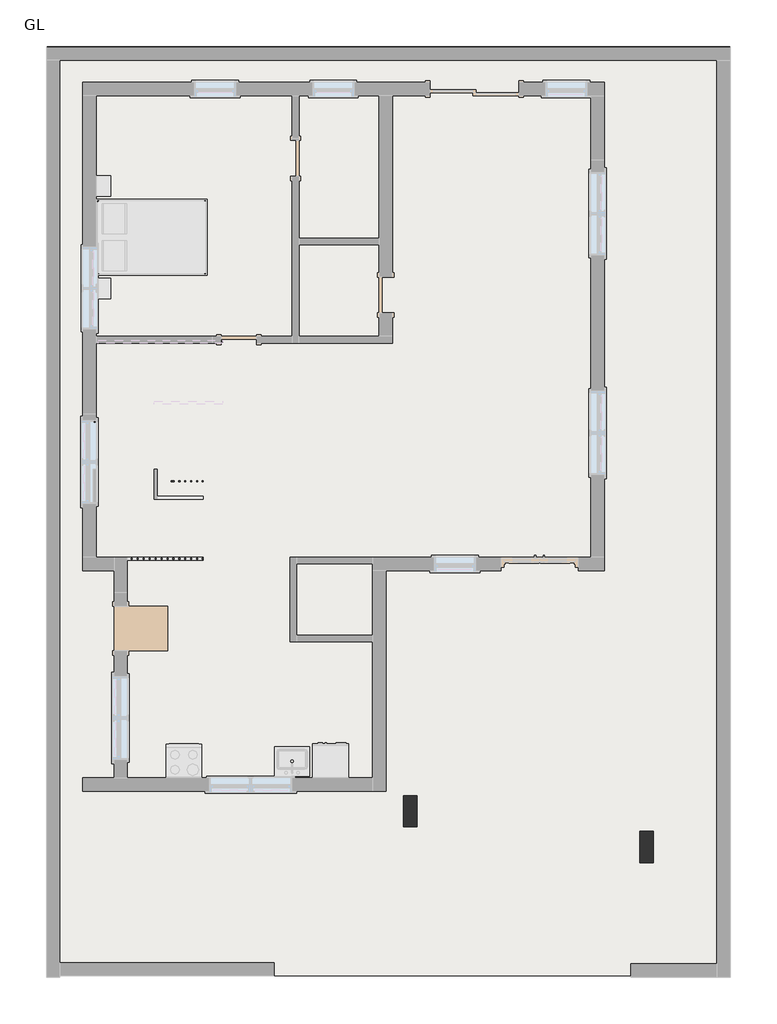
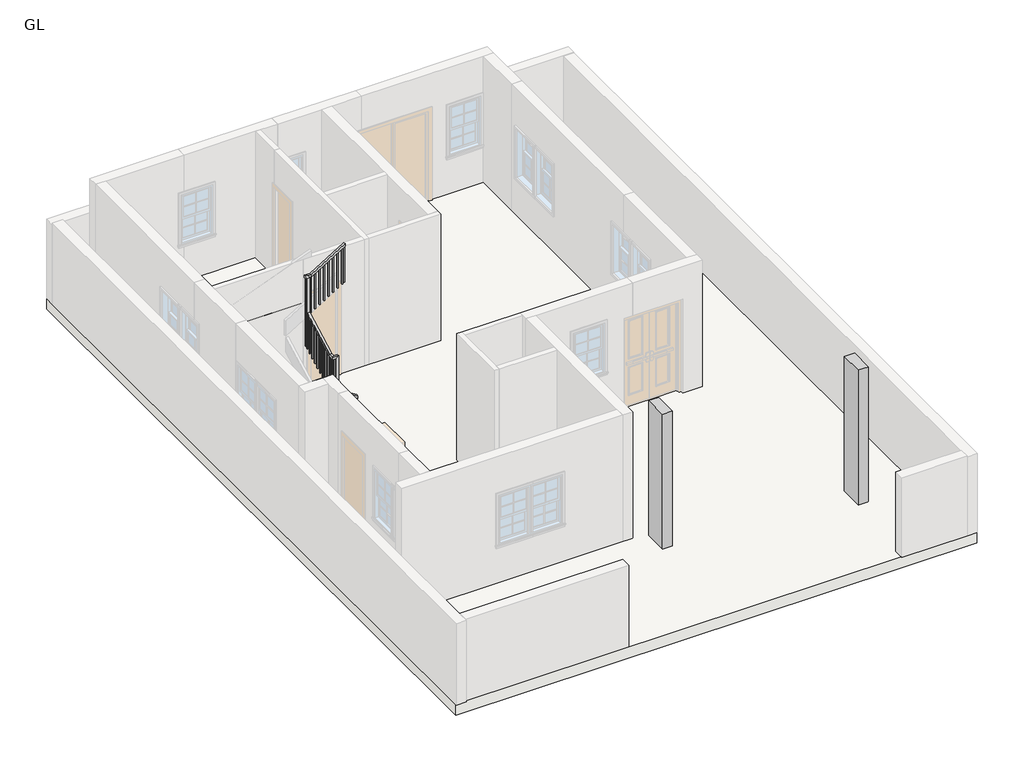
# One storey, part 2 of 3: 2 columns, 2 railings, 1 slab.
"""IFC4 building model written with IfcOpenShell, lengths in millimetres."""

from ifc_helpers import new_model, si_unit, frame, origin, place, context, project, spatial, polyline, outline, extrude, faceted_brep, transform, mapped, element, save
from components import column_1de33f28

model = new_model("IFC4")

# Units and contexts
model_context = context("Model", 3, world=origin())
ifc_project = project(units=[si_unit("LENGTHUNIT", "METRE", prefix="MILLI")], contexts=[model_context])

# Site, building, storey
site = spatial("IfcSite", under=ifc_project)
building = spatial("IfcBuilding", under=site)
storey = spatial("IfcBuildingStorey", under=building, Name="GL", Elevation=0.0)

# Columns
placement = place(None, origin())
column_shape = column_1de33f28(model_context)
element("IfcColumn", 1, ObjectType="Rectangular Column : x9\"", at=placement, inside=storey, context=model_context, shape_type="MappedRepresentation", body=[
    mapped(column_shape, transform((-16875.4750314, 319.9223646, 0.0), x_axis=(1.0, 0.0, 0.0), y_axis=(0.0, 1.0, 0.0), z_axis=(0.0, 0.0, 1.0))),
])
element("IfcColumn", 2, ObjectType="Rectangular Column : x9\"", at=placement, inside=storey, context=model_context, shape_type="MappedRepresentation", body=[
    mapped(column_shape, transform((-12836.8750314, -289.6776354, 0.0), x_axis=(1.0, 0.0, 0.0), y_axis=(0.0, 1.0, 0.0), z_axis=(0.0, 0.0, 1.0))),
])

# Railings
element("IfcRailing", 3, ObjectType="Handrail - Rectangular", at=placement, inside=storey, context=model_context, shape_type="SolidModel", body=[
    faceted_brep([(-20418.7750314, 5933.3223646, 1270.0), (-20418.7750314, 5933.3223646, 1209.786276), (-20418.7750314, 5984.1223646, 1209.786276), (-20418.7750314, 5984.1223646, 1270.0), (-20850.5750314, 5933.3223646, 1544.7818182), (-20901.3750314, 5933.3223646, 1516.8953669), (-20901.3750314, 5984.1223646, 1516.8953669), (-20850.5750314, 5984.1223646, 1544.7818182), (-20850.5750314, 5933.3223646, 2374.5151515), (-20901.3750314, 5933.3223646, 2323.7151515), (-20901.3750314, 5984.1223646, 2323.7151515), (-20850.5750314, 5984.1223646, 2374.5151515), (-20977.5750314, 5933.3223646, 2374.5151515), (-20977.5750314, 5933.3223646, 2323.7151515), (-20926.7750314, 5984.1223646, 2323.7151515), (-20926.7750314, 5984.1223646, 2374.5151515), (-20977.5750314, 6060.3223646, 2374.5151515), (-20977.5750314, 6072.9586335, 2323.7151515), (-20926.7750314, 6072.9586335, 2323.7151515), (-20926.7750314, 6060.3223646, 2374.5151515), (-20977.5750314, 6923.9223646, 2832.4848485), (-20977.5750314, 6974.7223646, 2801.9231907), (-20926.7750314, 6974.7223646, 2801.9231907), (-20926.7750314, 6923.9223646, 2832.4848485), (-20088.5750314, 7050.9223646, 4114.8), (-20088.5750314, 7000.1223646, 4114.8), (-20088.5750314, 7000.1223646, 4055.3290495), (-20088.5750314, 7050.9223646, 4055.3290495), (-20836.3298984, 7050.9223646, 3600.173913), (-20850.5750314, 7050.9223646, 3650.973913), (-20836.3298984, 7000.1223646, 3600.173913), (-20850.5750314, 7000.1223646, 3650.973913), (-20977.5750314, 6923.9223646, 3650.973913), (-20977.5750314, 6974.7223646, 3600.173913), (-20926.7750314, 6974.7223646, 3600.173913), (-20926.7750314, 6923.9223646, 3650.973913), (-20977.5750314, 7050.9223646, 3650.973913), (-20977.5750314, 7050.9223646, 3600.173913), (-20926.7750314, 7000.1223646, 3600.173913), (-20926.7750314, 7000.1223646, 3650.973913)], [[[0, 1, 2, 3]], [[1, 0, 4, 5]], [[2, 1, 5, 6]], [[3, 2, 6, 7]], [[0, 3, 7, 4]], [[5, 4, 8, 9]], [[6, 5, 9, 10]], [[7, 6, 10, 11]], [[4, 7, 11, 8]], [[9, 8, 12, 13]], [[10, 9, 13, 14]], [[11, 10, 14, 15]], [[8, 11, 15, 12]], [[13, 12, 16, 17]], [[14, 13, 17, 18]], [[15, 14, 18, 19]], [[12, 15, 19, 16]], [[17, 16, 20, 21]], [[18, 17, 21, 22]], [[19, 18, 22, 23]], [[16, 19, 23, 20]], [[24, 25, 26, 27]], [[28, 29, 24, 27]], [[30, 28, 27, 26]], [[31, 30, 26, 25]], [[29, 31, 25, 24]], [[21, 20, 32, 33]], [[22, 21, 33, 34]], [[23, 22, 34, 35]], [[20, 23, 35, 32]], [[33, 32, 36, 37]], [[34, 33, 37, 38]], [[35, 34, 38, 39]], [[32, 35, 39, 36]], [[37, 36, 29, 28]], [[38, 37, 28, 30]], [[39, 38, 30, 31]], [[36, 39, 31, 29]]]),
    extrude(outline(polyline([(4030.2051365, -20129.8500314), (4018.6094843, -20148.9000314), (3169.4782609, -20148.9000314), (3169.4782609, -20129.8500314), (4030.2051365, -20129.8500314)])), frame((0.0, 7015.9973646, 0.0), z_axis=(0.0, 1.0, 0.0), x_axis=(0.0, 0.0, 1.0)), (0.0, 0.0, 1.0), 19.05),
    extrude(outline(polyline([(3968.3616582, -20231.4500314), (3956.766006, -20250.5000314), (3107.6347826, -20250.5000314), (3107.6347826, -20231.4500314), (3968.3616582, -20231.4500314)])), frame((0.0, 7015.9973646, 0.0), z_axis=(0.0, 1.0, 0.0), x_axis=(0.0, 0.0, 1.0)), (0.0, 0.0, 1.0), 19.05),
    extrude(outline(polyline([(3906.51818, -20333.0500314), (3894.9225278, -20352.1000314), (3045.7913043, -20352.1000314), (3045.7913043, -20333.0500314), (3906.51818, -20333.0500314)])), frame((0.0, 7015.9973646, 0.0), z_axis=(0.0, 1.0, 0.0), x_axis=(0.0, 0.0, 1.0)), (0.0, 0.0, 1.0), 19.05),
    extrude(outline(polyline([(3844.6747017, -20434.6500314), (3833.0790495, -20453.7000314), (2983.9478261, -20453.7000314), (2983.9478261, -20434.6500314), (3844.6747017, -20434.6500314)])), frame((0.0, 7015.9973646, 0.0), z_axis=(0.0, 1.0, 0.0), x_axis=(0.0, 0.0, 1.0)), (0.0, 0.0, 1.0), 19.05),
    extrude(outline(polyline([(3782.8312234, -20536.2500314), (3771.2355713, -20555.3000314), (2922.1043478, -20555.3000314), (2922.1043478, -20536.2500314), (3782.8312234, -20536.2500314)])), frame((0.0, 7015.9973646, 0.0), z_axis=(0.0, 1.0, 0.0), x_axis=(0.0, 0.0, 1.0)), (0.0, 0.0, 1.0), 19.05),
    extrude(outline(polyline([(3720.9877452, -20637.8500314), (3709.392093, -20656.9000314), (2860.2608696, -20656.9000314), (2860.2608696, -20637.8500314), (3720.9877452, -20637.8500314)])), frame((0.0, 7015.9973646, 0.0), z_axis=(0.0, 1.0, 0.0), x_axis=(0.0, 0.0, 1.0)), (0.0, 0.0, 1.0), 19.05),
    extrude(outline(polyline([(3659.1442669, -20739.4500314), (3647.5486147, -20758.5000314), (2798.4173913, -20758.5000314), (2798.4173913, -20739.4500314), (3659.1442669, -20739.4500314)])), frame((0.0, 7015.9973646, 0.0), z_axis=(0.0, 1.0, 0.0), x_axis=(0.0, 0.0, 1.0)), (0.0, 0.0, 1.0), 19.05),
    extrude(outline(polyline([(3597.3007887, -20841.0500314), (3585.7051365, -20860.1000314), (2736.573913, -20860.1000314), (2736.573913, -20841.0500314), (3597.3007887, -20841.0500314)])), frame((0.0, 7015.9973646, 0.0), z_axis=(0.0, 1.0, 0.0), x_axis=(0.0, 0.0, 1.0)), (0.0, 0.0, 1.0), 19.05),
    extrude(outline(polyline([(-20942.6500314, 6965.1973646), (-20961.7000314, 6965.1973646), (-20961.7000314, 6984.2473646), (-20942.6500314, 6984.2473646), (-20942.6500314, 6965.1973646)])), frame((0.0, 0.0, 1945.0242424), z_axis=(0.0, 0.0, 1.0), x_axis=(1.0, 0.0, 0.0)), (0.0, 0.0, 1.0), 1655.1496706),
    extrude(outline(polyline([(6863.5973646, 2742.9932665), (6882.6473646, 2753.0955392), (6882.6473646, 1891.1454545), (6863.5973646, 1891.1454545), (6863.5973646, 2742.9932665)])), frame((-20961.7000314, 0.0, 0.0), z_axis=(1.0, 0.0, 0.0), x_axis=(0.0, 1.0, 0.0)), (0.0, 0.0, 1.0), 19.05),
    extrude(outline(polyline([(6761.9973646, 2689.1144786), (6781.0473646, 2699.2167513), (6781.0473646, 1837.2666667), (6761.9973646, 1837.2666667), (6761.9973646, 2689.1144786)])), frame((-20961.7000314, 0.0, 0.0), z_axis=(1.0, 0.0, 0.0), x_axis=(0.0, 1.0, 0.0)), (0.0, 0.0, 1.0), 19.05),
    extrude(outline(polyline([(6660.3973646, 2635.2356907), (6679.4473646, 2645.3379635), (6679.4473646, 1783.3878788), (6660.3973646, 1783.3878788), (6660.3973646, 2635.2356907)])), frame((-20961.7000314, 0.0, 0.0), z_axis=(1.0, 0.0, 0.0), x_axis=(0.0, 1.0, 0.0)), (0.0, 0.0, 1.0), 19.05),
    extrude(outline(polyline([(6558.7973646, 2581.3569029), (6577.8473646, 2591.4591756), (6577.8473646, 1729.5090909), (6558.7973646, 1729.5090909), (6558.7973646, 2581.3569029)])), frame((-20961.7000314, 0.0, 0.0), z_axis=(1.0, 0.0, 0.0), x_axis=(0.0, 1.0, 0.0)), (0.0, 0.0, 1.0), 19.05),
    extrude(outline(polyline([(6457.1973646, 2527.478115), (6476.2473646, 2537.5803877), (6476.2473646, 1675.630303), (6457.1973646, 1675.630303), (6457.1973646, 2527.478115)])), frame((-20961.7000314, 0.0, 0.0), z_axis=(1.0, 0.0, 0.0), x_axis=(0.0, 1.0, 0.0)), (0.0, 0.0, 1.0), 19.05),
    extrude(outline(polyline([(6355.5973646, 2473.5993271), (6374.6473646, 2483.7015998), (6374.6473646, 1621.7515152), (6355.5973646, 1621.7515152), (6355.5973646, 2473.5993271)])), frame((-20961.7000314, 0.0, 0.0), z_axis=(1.0, 0.0, 0.0), x_axis=(0.0, 1.0, 0.0)), (0.0, 0.0, 1.0), 19.05),
    extrude(outline(polyline([(6253.9973646, 2419.7205392), (6273.0473646, 2429.8228119), (6273.0473646, 1567.8727273), (6253.9973646, 1567.8727273), (6253.9973646, 2419.7205392)])), frame((-20961.7000314, 0.0, 0.0), z_axis=(1.0, 0.0, 0.0), x_axis=(0.0, 1.0, 0.0)), (0.0, 0.0, 1.0), 19.05),
    extrude(outline(polyline([(6152.3973646, 2365.8417513), (6171.4473646, 2375.9440241), (6171.4473646, 1513.9939394), (6152.3973646, 1513.9939394), (6152.3973646, 2365.8417513)])), frame((-20961.7000314, 0.0, 0.0), z_axis=(1.0, 0.0, 0.0), x_axis=(0.0, 1.0, 0.0)), (0.0, 0.0, 1.0), 19.05),
    extrude(outline(polyline([(6050.7973646, 2311.9629635), (6069.8473646, 2322.0652362), (6069.8473646, 1460.1151515), (6050.7973646, 1460.1151515), (6050.7973646, 2311.9629635)])), frame((-20961.7000314, 0.0, 0.0), z_axis=(1.0, 0.0, 0.0), x_axis=(0.0, 1.0, 0.0)), (0.0, 0.0, 1.0), 19.05),
    extrude(outline(polyline([(-20917.2500314, 5968.2473646), (-20917.2500314, 5949.1973646), (-20936.3000314, 5949.1973646), (-20936.3000314, 5968.2473646), (-20917.2500314, 5968.2473646)])), frame((0.0, 0.0, 678.8727273), z_axis=(0.0, 0.0, 1.0), x_axis=(1.0, 0.0, 0.0)), (0.0, 0.0, 1.0), 1644.8424242),
    extrude(outline(polyline([(1462.3430941, -20815.6500314), (1474.4658214, -20834.7000314), (614.2181818, -20834.7000314), (614.2181818, -20815.6500314), (1462.3430941, -20815.6500314)])), frame((0.0, 5949.1973646, 0.0), z_axis=(0.0, 1.0, 0.0), x_axis=(0.0, 0.0, 1.0)), (0.0, 0.0, 1.0), 19.05),
    extrude(outline(polyline([(1397.6885487, -20714.0500314), (1409.811276, -20733.1000314), (549.5636364, -20733.1000314), (549.5636364, -20714.0500314), (1397.6885487, -20714.0500314)])), frame((0.0, 5949.1973646, 0.0), z_axis=(0.0, 1.0, 0.0), x_axis=(0.0, 0.0, 1.0)), (0.0, 0.0, 1.0), 19.05),
    extrude(outline(polyline([(1333.0340032, -20612.4500314), (1345.1567305, -20631.5000314), (484.9090909, -20631.5000314), (484.9090909, -20612.4500314), (1333.0340032, -20612.4500314)])), frame((0.0, 5949.1973646, 0.0), z_axis=(0.0, 1.0, 0.0), x_axis=(0.0, 0.0, 1.0)), (0.0, 0.0, 1.0), 19.05),
    extrude(outline(polyline([(1268.3794578, -20510.8500314), (1280.5021851, -20529.9000314), (420.2545455, -20529.9000314), (420.2545455, -20510.8500314), (1268.3794578, -20510.8500314)])), frame((0.0, 5949.1973646, 0.0), z_axis=(0.0, 1.0, 0.0), x_axis=(0.0, 0.0, 1.0)), (0.0, 0.0, 1.0), 19.05),
    extrude(outline(polyline([(-20942.6500314, 7015.9973646), (-20961.7000314, 7015.9973646), (-20961.7000314, 7035.0473646), (-20942.6500314, 7035.0473646), (-20942.6500314, 7015.9973646)])), frame((0.0, 0.0, 1971.9636364), z_axis=(0.0, 0.0, 1.0), x_axis=(1.0, 0.0, 0.0)), (0.0, 0.0, 1.0), 1628.2102767),
    extrude(outline(polyline([(-20942.6500314, 5968.2473646), (-20942.6500314, 5949.1973646), (-20961.7000314, 5949.1973646), (-20961.7000314, 5968.2473646), (-20942.6500314, 5968.2473646)])), frame((0.0, 0.0, 695.0363636), z_axis=(0.0, 0.0, 1.0), x_axis=(1.0, 0.0, 0.0)), (0.0, 0.0, 1.0), 1628.6787879),
    extrude(outline(polyline([(4055.3290495, -20088.5750314), (4043.7333973, -20107.6250314), (3194.6021739, -20107.6250314), (3194.6021739, -20088.5750314), (4055.3290495, -20088.5750314)])), frame((0.0, 7015.9973646, 0.0), z_axis=(0.0, 1.0, 0.0), x_axis=(0.0, 0.0, 1.0)), (0.0, 0.0, 1.0), 19.05),
    extrude(outline(polyline([(1209.786276, -20418.7750314), (1221.9090032, -20437.8250314), (361.6613636, -20437.8250314), (361.6613636, -20418.7750314), (1209.786276, -20418.7750314)])), frame((0.0, 5949.1973646, 0.0), z_axis=(0.0, 1.0, 0.0), x_axis=(0.0, 0.0, 1.0)), (0.0, 0.0, 1.0), 19.05),
])
element("IfcRailing", 4, ObjectType="Handrail - Rectangular", at=placement, inside=storey, context=model_context, shape_type="SolidModel", body=[
    faceted_brep([(-20418.7750314, 4612.5223646, 1270.0), (-20418.7750314, 4612.5223646, 1215.4938354), (-20418.7750314, 4663.3223646, 1215.4938354), (-20418.7750314, 4663.3223646, 1270.0), (-22171.3752061, 4612.5223646, 1951.5667346), (-22222.1752061, 4612.5223646, 1916.8161256), (-22222.1752061, 4663.3223646, 1916.8161256), (-22171.3752061, 4663.3223646, 1951.5667346), (-22171.3752061, 4612.5223646, 1981.200068), (-22222.1752061, 4612.5223646, 1930.400068), (-22222.1752061, 4663.3223646, 1930.400068), (-22171.3752061, 4663.3223646, 1981.200068), (-22298.3752061, 4612.5223646, 1981.200068), (-22298.3752061, 4612.5223646, 1930.400068), (-22247.5752061, 4663.3223646, 1930.400068), (-22247.5752061, 4663.3223646, 1981.200068), (-22298.3752061, 4739.5223646, 1981.200068), (-22298.3752061, 4739.5223646, 1930.400068), (-22247.5752061, 4739.5223646, 1930.400068), (-22247.5752061, 4739.5223646, 1981.200068), (-22298.3752061, 8371.7223646, 1981.200068), (-22298.3752061, 8371.7223646, 1930.400068), (-22247.5752061, 8320.9223646, 1930.400068), (-22247.5752061, 8320.9223646, 1981.200068), (-20088.5750314, 8371.7223646, 1981.200068), (-20088.5750314, 8320.9223646, 1981.200068), (-20088.5750314, 8320.9223646, 1930.400068), (-20088.5750314, 8371.7223646, 1930.400068)], [[[0, 1, 2, 3]], [[1, 0, 4, 5]], [[2, 1, 5, 6]], [[3, 2, 6, 7]], [[0, 3, 7, 4]], [[5, 4, 8, 9]], [[6, 5, 9, 10]], [[7, 6, 10, 11]], [[4, 7, 11, 8]], [[9, 8, 12, 13]], [[10, 9, 13, 14]], [[11, 10, 14, 15]], [[8, 11, 15, 12]], [[13, 12, 16, 17]], [[14, 13, 17, 18]], [[15, 14, 18, 19]], [[12, 15, 19, 16]], [[17, 16, 20, 21]], [[18, 17, 21, 22]], [[19, 18, 22, 23]], [[16, 19, 23, 20]], [[24, 25, 26, 27]], [[21, 20, 24, 27]], [[22, 21, 27, 26]], [[23, 22, 26, 25]], [[20, 23, 25, 24]]]),
    extrude(outline(polyline([(-20148.9002061, 8355.8473646), (-20129.8502061, 8355.8473646), (-20129.8502061, 8336.7973646), (-20148.9002061, 8336.7973646), (-20148.9002061, 8355.8473646)])), frame((0.0, 0.0, 1066.800068), z_axis=(0.0, 0.0, 1.0), x_axis=(1.0, 0.0, 0.0)), (0.0, 0.0, 1.0), 863.6),
    extrude(outline(polyline([(-20250.5002061, 8355.8473646), (-20231.4502061, 8355.8473646), (-20231.4502061, 8336.7973646), (-20250.5002061, 8336.7973646), (-20250.5002061, 8355.8473646)])), frame((0.0, 0.0, 1066.800068), z_axis=(0.0, 0.0, 1.0), x_axis=(1.0, 0.0, 0.0)), (0.0, 0.0, 1.0), 863.6),
    extrude(outline(polyline([(-20352.1002061, 8355.8473646), (-20333.0502061, 8355.8473646), (-20333.0502061, 8336.7973646), (-20352.1002061, 8336.7973646), (-20352.1002061, 8355.8473646)])), frame((0.0, 0.0, 1066.800068), z_axis=(0.0, 0.0, 1.0), x_axis=(1.0, 0.0, 0.0)), (0.0, 0.0, 1.0), 863.6),
    extrude(outline(polyline([(-20453.7002061, 8355.8473646), (-20434.6502061, 8355.8473646), (-20434.6502061, 8336.7973646), (-20453.7002061, 8336.7973646), (-20453.7002061, 8355.8473646)])), frame((0.0, 0.0, 1066.800068), z_axis=(0.0, 0.0, 1.0), x_axis=(1.0, 0.0, 0.0)), (0.0, 0.0, 1.0), 863.6),
    extrude(outline(polyline([(-20555.3002061, 8355.8473646), (-20536.2502061, 8355.8473646), (-20536.2502061, 8336.7973646), (-20555.3002061, 8336.7973646), (-20555.3002061, 8355.8473646)])), frame((0.0, 0.0, 1066.800068), z_axis=(0.0, 0.0, 1.0), x_axis=(1.0, 0.0, 0.0)), (0.0, 0.0, 1.0), 863.6),
    extrude(outline(polyline([(-20656.9002061, 8355.8473646), (-20637.8502061, 8355.8473646), (-20637.8502061, 8336.7973646), (-20656.9002061, 8336.7973646), (-20656.9002061, 8355.8473646)])), frame((0.0, 0.0, 1066.800068), z_axis=(0.0, 0.0, 1.0), x_axis=(1.0, 0.0, 0.0)), (0.0, 0.0, 1.0), 863.6),
    extrude(outline(polyline([(-20758.5002061, 8355.8473646), (-20739.4502061, 8355.8473646), (-20739.4502061, 8336.7973646), (-20758.5002061, 8336.7973646), (-20758.5002061, 8355.8473646)])), frame((0.0, 0.0, 1066.800068), z_axis=(0.0, 0.0, 1.0), x_axis=(1.0, 0.0, 0.0)), (0.0, 0.0, 1.0), 863.6),
    extrude(outline(polyline([(-20860.1002061, 8355.8473646), (-20841.0502061, 8355.8473646), (-20841.0502061, 8336.7973646), (-20860.1002061, 8336.7973646), (-20860.1002061, 8355.8473646)])), frame((0.0, 0.0, 1066.800068), z_axis=(0.0, 0.0, 1.0), x_axis=(1.0, 0.0, 0.0)), (0.0, 0.0, 1.0), 863.6),
    extrude(outline(polyline([(-20961.7002061, 8355.8473646), (-20942.6502061, 8355.8473646), (-20942.6502061, 8336.7973646), (-20961.7002061, 8336.7973646), (-20961.7002061, 8355.8473646)])), frame((0.0, 0.0, 1066.800068), z_axis=(0.0, 0.0, 1.0), x_axis=(1.0, 0.0, 0.0)), (0.0, 0.0, 1.0), 863.6),
    extrude(outline(polyline([(-21063.3002061, 8355.8473646), (-21044.2502061, 8355.8473646), (-21044.2502061, 8336.7973646), (-21063.3002061, 8336.7973646), (-21063.3002061, 8355.8473646)])), frame((0.0, 0.0, 1066.800068), z_axis=(0.0, 0.0, 1.0), x_axis=(1.0, 0.0, 0.0)), (0.0, 0.0, 1.0), 863.6),
    extrude(outline(polyline([(-21164.9002061, 8355.8473646), (-21145.8502061, 8355.8473646), (-21145.8502061, 8336.7973646), (-21164.9002061, 8336.7973646), (-21164.9002061, 8355.8473646)])), frame((0.0, 0.0, 1066.800068), z_axis=(0.0, 0.0, 1.0), x_axis=(1.0, 0.0, 0.0)), (0.0, 0.0, 1.0), 863.6),
    extrude(outline(polyline([(-21266.5002061, 8355.8473646), (-21247.4502061, 8355.8473646), (-21247.4502061, 8336.7973646), (-21266.5002061, 8336.7973646), (-21266.5002061, 8355.8473646)])), frame((0.0, 0.0, 1066.800068), z_axis=(0.0, 0.0, 1.0), x_axis=(1.0, 0.0, 0.0)), (0.0, 0.0, 1.0), 863.6),
    extrude(outline(polyline([(-21368.1002061, 8355.8473646), (-21349.0502061, 8355.8473646), (-21349.0502061, 8336.7973646), (-21368.1002061, 8336.7973646), (-21368.1002061, 8355.8473646)])), frame((0.0, 0.0, 1066.800068), z_axis=(0.0, 0.0, 1.0), x_axis=(1.0, 0.0, 0.0)), (0.0, 0.0, 1.0), 863.6),
    extrude(outline(polyline([(-21469.7002061, 8355.8473646), (-21450.6502061, 8355.8473646), (-21450.6502061, 8336.7973646), (-21469.7002061, 8336.7973646), (-21469.7002061, 8355.8473646)])), frame((0.0, 0.0, 1066.800068), z_axis=(0.0, 0.0, 1.0), x_axis=(1.0, 0.0, 0.0)), (0.0, 0.0, 1.0), 863.6),
    extrude(outline(polyline([(-21571.3002061, 8355.8473646), (-21552.2502061, 8355.8473646), (-21552.2502061, 8336.7973646), (-21571.3002061, 8336.7973646), (-21571.3002061, 8355.8473646)])), frame((0.0, 0.0, 1066.800068), z_axis=(0.0, 0.0, 1.0), x_axis=(1.0, 0.0, 0.0)), (0.0, 0.0, 1.0), 863.6),
    extrude(outline(polyline([(-21672.9002061, 8355.8473646), (-21653.8502061, 8355.8473646), (-21653.8502061, 8336.7973646), (-21672.9002061, 8336.7973646), (-21672.9002061, 8355.8473646)])), frame((0.0, 0.0, 1066.800068), z_axis=(0.0, 0.0, 1.0), x_axis=(1.0, 0.0, 0.0)), (0.0, 0.0, 1.0), 863.6),
    extrude(outline(polyline([(-21774.5002061, 8355.8473646), (-21755.4502061, 8355.8473646), (-21755.4502061, 8336.7973646), (-21774.5002061, 8336.7973646), (-21774.5002061, 8355.8473646)])), frame((0.0, 0.0, 1066.800068), z_axis=(0.0, 0.0, 1.0), x_axis=(1.0, 0.0, 0.0)), (0.0, 0.0, 1.0), 863.6),
    extrude(outline(polyline([(-21876.1002061, 8355.8473646), (-21857.0502061, 8355.8473646), (-21857.0502061, 8336.7973646), (-21876.1002061, 8336.7973646), (-21876.1002061, 8355.8473646)])), frame((0.0, 0.0, 1066.800068), z_axis=(0.0, 0.0, 1.0), x_axis=(1.0, 0.0, 0.0)), (0.0, 0.0, 1.0), 863.6),
    extrude(outline(polyline([(-21977.7002061, 8355.8473646), (-21958.6502061, 8355.8473646), (-21958.6502061, 8336.7973646), (-21977.7002061, 8336.7973646), (-21977.7002061, 8355.8473646)])), frame((0.0, 0.0, 1066.800068), z_axis=(0.0, 0.0, 1.0), x_axis=(1.0, 0.0, 0.0)), (0.0, 0.0, 1.0), 863.6),
    extrude(outline(polyline([(-22079.3002061, 8355.8473646), (-22060.2502061, 8355.8473646), (-22060.2502061, 8336.7973646), (-22079.3002061, 8336.7973646), (-22079.3002061, 8355.8473646)])), frame((0.0, 0.0, 1066.800068), z_axis=(0.0, 0.0, 1.0), x_axis=(1.0, 0.0, 0.0)), (0.0, 0.0, 1.0), 863.6),
    extrude(outline(polyline([(-22180.9002061, 8355.8473646), (-22161.8502061, 8355.8473646), (-22161.8502061, 8336.7973646), (-22180.9002061, 8336.7973646), (-22180.9002061, 8355.8473646)])), frame((0.0, 0.0, 1066.800068), z_axis=(0.0, 0.0, 1.0), x_axis=(1.0, 0.0, 0.0)), (0.0, 0.0, 1.0), 863.6),
    extrude(outline(polyline([(-22282.5002061, 8285.9973646), (-22282.5002061, 8305.0473646), (-22263.4502061, 8305.0473646), (-22263.4502061, 8285.9973646), (-22282.5002061, 8285.9973646)])), frame((0.0, 0.0, 1066.800068), z_axis=(0.0, 0.0, 1.0), x_axis=(1.0, 0.0, 0.0)), (0.0, 0.0, 1.0), 863.6),
    extrude(outline(polyline([(-22282.5002061, 8184.3973646), (-22282.5002061, 8203.4473646), (-22263.4502061, 8203.4473646), (-22263.4502061, 8184.3973646), (-22282.5002061, 8184.3973646)])), frame((0.0, 0.0, 1066.800068), z_axis=(0.0, 0.0, 1.0), x_axis=(1.0, 0.0, 0.0)), (0.0, 0.0, 1.0), 863.6),
    extrude(outline(polyline([(-22282.5002061, 8082.7973646), (-22282.5002061, 8101.8473646), (-22263.4502061, 8101.8473646), (-22263.4502061, 8082.7973646), (-22282.5002061, 8082.7973646)])), frame((0.0, 0.0, 1066.800068), z_axis=(0.0, 0.0, 1.0), x_axis=(1.0, 0.0, 0.0)), (0.0, 0.0, 1.0), 863.6),
    extrude(outline(polyline([(-22282.5002061, 7981.1973646), (-22282.5002061, 8000.2473646), (-22263.4502061, 8000.2473646), (-22263.4502061, 7981.1973646), (-22282.5002061, 7981.1973646)])), frame((0.0, 0.0, 1066.800068), z_axis=(0.0, 0.0, 1.0), x_axis=(1.0, 0.0, 0.0)), (0.0, 0.0, 1.0), 863.6),
    extrude(outline(polyline([(-22282.5002061, 7879.5973646), (-22282.5002061, 7898.6473646), (-22263.4502061, 7898.6473646), (-22263.4502061, 7879.5973646), (-22282.5002061, 7879.5973646)])), frame((0.0, 0.0, 1066.800068), z_axis=(0.0, 0.0, 1.0), x_axis=(1.0, 0.0, 0.0)), (0.0, 0.0, 1.0), 863.6),
    extrude(outline(polyline([(-22282.5002061, 7777.9973646), (-22282.5002061, 7797.0473646), (-22263.4502061, 7797.0473646), (-22263.4502061, 7777.9973646), (-22282.5002061, 7777.9973646)])), frame((0.0, 0.0, 1066.800068), z_axis=(0.0, 0.0, 1.0), x_axis=(1.0, 0.0, 0.0)), (0.0, 0.0, 1.0), 863.6),
    extrude(outline(polyline([(-22282.5002061, 7676.3973646), (-22282.5002061, 7695.4473646), (-22263.4502061, 7695.4473646), (-22263.4502061, 7676.3973646), (-22282.5002061, 7676.3973646)])), frame((0.0, 0.0, 1066.800068), z_axis=(0.0, 0.0, 1.0), x_axis=(1.0, 0.0, 0.0)), (0.0, 0.0, 1.0), 863.6),
    extrude(outline(polyline([(-22282.5002061, 7574.7973646), (-22282.5002061, 7593.8473646), (-22263.4502061, 7593.8473646), (-22263.4502061, 7574.7973646), (-22282.5002061, 7574.7973646)])), frame((0.0, 0.0, 1066.800068), z_axis=(0.0, 0.0, 1.0), x_axis=(1.0, 0.0, 0.0)), (0.0, 0.0, 1.0), 863.6),
    extrude(outline(polyline([(-22282.5002061, 7473.1973646), (-22282.5002061, 7492.2473646), (-22263.4502061, 7492.2473646), (-22263.4502061, 7473.1973646), (-22282.5002061, 7473.1973646)])), frame((0.0, 0.0, 1066.800068), z_axis=(0.0, 0.0, 1.0), x_axis=(1.0, 0.0, 0.0)), (0.0, 0.0, 1.0), 863.6),
    extrude(outline(polyline([(-22282.5002061, 7371.5973646), (-22282.5002061, 7390.6473646), (-22263.4502061, 7390.6473646), (-22263.4502061, 7371.5973646), (-22282.5002061, 7371.5973646)])), frame((0.0, 0.0, 1066.800068), z_axis=(0.0, 0.0, 1.0), x_axis=(1.0, 0.0, 0.0)), (0.0, 0.0, 1.0), 863.6),
    extrude(outline(polyline([(-22282.5002061, 7269.9973646), (-22282.5002061, 7289.0473646), (-22263.4502061, 7289.0473646), (-22263.4502061, 7269.9973646), (-22282.5002061, 7269.9973646)])), frame((0.0, 0.0, 1066.800068), z_axis=(0.0, 0.0, 1.0), x_axis=(1.0, 0.0, 0.0)), (0.0, 0.0, 1.0), 863.6),
    extrude(outline(polyline([(-22282.5002061, 7168.3973646), (-22282.5002061, 7187.4473646), (-22263.4502061, 7187.4473646), (-22263.4502061, 7168.3973646), (-22282.5002061, 7168.3973646)])), frame((0.0, 0.0, 1066.800068), z_axis=(0.0, 0.0, 1.0), x_axis=(1.0, 0.0, 0.0)), (0.0, 0.0, 1.0), 863.6),
    extrude(outline(polyline([(-22282.5002061, 7066.7973646), (-22282.5002061, 7085.8473646), (-22263.4502061, 7085.8473646), (-22263.4502061, 7066.7973646), (-22282.5002061, 7066.7973646)])), frame((0.0, 0.0, 1066.800068), z_axis=(0.0, 0.0, 1.0), x_axis=(1.0, 0.0, 0.0)), (0.0, 0.0, 1.0), 863.6),
    extrude(outline(polyline([(-22282.5002061, 6965.1973646), (-22282.5002061, 6984.2473646), (-22263.4502061, 6984.2473646), (-22263.4502061, 6965.1973646), (-22282.5002061, 6965.1973646)])), frame((0.0, 0.0, 1066.800068), z_axis=(0.0, 0.0, 1.0), x_axis=(1.0, 0.0, 0.0)), (0.0, 0.0, 1.0), 863.6),
    extrude(outline(polyline([(6882.6473646, 1930.400068), (6882.6473646, 1923.8894652), (6863.5973646, 1913.7871925), (6863.5973646, 1930.400068), (6882.6473646, 1930.400068)])), frame((-22282.5002061, 0.0, 0.0), z_axis=(1.0, 0.0, 0.0), x_axis=(0.0, 1.0, 0.0)), (0.0, 0.0, 1.0), 19.05),
    extrude(outline(polyline([(6781.0473646, 1930.400068), (6781.0473646, 1870.0106774), (6761.9973646, 1859.9084046), (6761.9973646, 1930.400068), (6781.0473646, 1930.400068)])), frame((-22282.5002061, 0.0, 0.0), z_axis=(1.0, 0.0, 0.0), x_axis=(0.0, 1.0, 0.0)), (0.0, 0.0, 1.0), 19.05),
    extrude(outline(polyline([(6679.4473646, 1930.400068), (6679.4473646, 1816.1318895), (6660.3973646, 1806.0296168), (6660.3973646, 1930.400068), (6679.4473646, 1930.400068)])), frame((-22282.5002061, 0.0, 0.0), z_axis=(1.0, 0.0, 0.0), x_axis=(0.0, 1.0, 0.0)), (0.0, 0.0, 1.0), 19.05),
    extrude(outline(polyline([(6577.8473646, 1930.400068), (6577.8473646, 1762.2531016), (6558.7973646, 1752.1508289), (6558.7973646, 1930.400068), (6577.8473646, 1930.400068)])), frame((-22282.5002061, 0.0, 0.0), z_axis=(1.0, 0.0, 0.0), x_axis=(0.0, 1.0, 0.0)), (0.0, 0.0, 1.0), 19.05),
    extrude(outline(polyline([(6476.2473646, 1930.400068), (6476.2473646, 1708.3743137), (6457.1973646, 1698.272041), (6457.1973646, 1930.400068), (6476.2473646, 1930.400068)])), frame((-22282.5002061, 0.0, 0.0), z_axis=(1.0, 0.0, 0.0), x_axis=(0.0, 1.0, 0.0)), (0.0, 0.0, 1.0), 19.05),
    extrude(outline(polyline([(6374.6473646, 1930.400068), (6374.6473646, 1654.4955258), (6355.5973646, 1644.3932531), (6355.5973646, 1930.400068), (6374.6473646, 1930.400068)])), frame((-22282.5002061, 0.0, 0.0), z_axis=(1.0, 0.0, 0.0), x_axis=(0.0, 1.0, 0.0)), (0.0, 0.0, 1.0), 19.05),
    extrude(outline(polyline([(6273.0473646, 1930.400068), (6273.0473646, 1600.616738), (6253.9973646, 1590.5144652), (6253.9973646, 1930.400068), (6273.0473646, 1930.400068)])), frame((-22282.5002061, 0.0, 0.0), z_axis=(1.0, 0.0, 0.0), x_axis=(0.0, 1.0, 0.0)), (0.0, 0.0, 1.0), 19.05),
    extrude(outline(polyline([(6171.4473646, 1930.400068), (6171.4473646, 1546.7379501), (6152.3973646, 1536.6356774), (6152.3973646, 1930.400068), (6171.4473646, 1930.400068)])), frame((-22282.5002061, 0.0, 0.0), z_axis=(1.0, 0.0, 0.0), x_axis=(0.0, 1.0, 0.0)), (0.0, 0.0, 1.0), 19.05),
    extrude(outline(polyline([(6069.8473646, 1930.400068), (6069.8473646, 1492.8591622), (6050.7973646, 1482.7568895), (6050.7973646, 1930.400068), (6069.8473646, 1930.400068)])), frame((-22282.5002061, 0.0, 0.0), z_axis=(1.0, 0.0, 0.0), x_axis=(0.0, 1.0, 0.0)), (0.0, 0.0, 1.0), 19.05),
    extrude(outline(polyline([(5968.2473646, 1930.400068), (5968.2473646, 1438.9803743), (5949.1973646, 1428.8781016), (5949.1973646, 1930.400068), (5968.2473646, 1930.400068)])), frame((-22282.5002061, 0.0, 0.0), z_axis=(1.0, 0.0, 0.0), x_axis=(0.0, 1.0, 0.0)), (0.0, 0.0, 1.0), 19.05),
    extrude(outline(polyline([(5866.6473646, 1930.400068), (5866.6473646, 1385.1015865), (5847.5973646, 1374.9993137), (5847.5973646, 1930.400068), (5866.6473646, 1930.400068)])), frame((-22282.5002061, 0.0, 0.0), z_axis=(1.0, 0.0, 0.0), x_axis=(0.0, 1.0, 0.0)), (0.0, 0.0, 1.0), 19.05),
    extrude(outline(polyline([(5765.0473646, 1930.400068), (5765.0473646, 1331.2227986), (5745.9973646, 1321.1205258), (5745.9973646, 1930.400068), (5765.0473646, 1930.400068)])), frame((-22282.5002061, 0.0, 0.0), z_axis=(1.0, 0.0, 0.0), x_axis=(0.0, 1.0, 0.0)), (0.0, 0.0, 1.0), 19.05),
    extrude(outline(polyline([(5663.4473646, 1930.400068), (5663.4473646, 1277.3440107), (5644.3973646, 1267.241738), (5644.3973646, 1930.400068), (5663.4473646, 1930.400068)])), frame((-22282.5002061, 0.0, 0.0), z_axis=(1.0, 0.0, 0.0), x_axis=(0.0, 1.0, 0.0)), (0.0, 0.0, 1.0), 19.05),
    extrude(outline(polyline([(5561.8473646, 1930.400068), (5561.8473646, 1223.4652228), (5542.7973646, 1213.3629501), (5542.7973646, 1930.400068), (5561.8473646, 1930.400068)])), frame((-22282.5002061, 0.0, 0.0), z_axis=(1.0, 0.0, 0.0), x_axis=(0.0, 1.0, 0.0)), (0.0, 0.0, 1.0), 19.05),
    extrude(outline(polyline([(5460.2473646, 1930.400068), (5460.2473646, 1169.5864349), (5441.1973646, 1159.4841622), (5441.1973646, 1930.400068), (5460.2473646, 1930.400068)])), frame((-22282.5002061, 0.0, 0.0), z_axis=(1.0, 0.0, 0.0), x_axis=(0.0, 1.0, 0.0)), (0.0, 0.0, 1.0), 19.05),
    extrude(outline(polyline([(5358.6473646, 1930.400068), (5358.6473646, 1115.7076471), (5339.5973646, 1105.6053743), (5339.5973646, 1930.400068), (5358.6473646, 1930.400068)])), frame((-22282.5002061, 0.0, 0.0), z_axis=(1.0, 0.0, 0.0), x_axis=(0.0, 1.0, 0.0)), (0.0, 0.0, 1.0), 19.05),
    extrude(outline(polyline([(5257.0473646, 1930.400068), (5257.0473646, 1061.8288592), (5237.9973646, 1051.7265865), (5237.9973646, 1930.400068), (5257.0473646, 1930.400068)])), frame((-22282.5002061, 0.0, 0.0), z_axis=(1.0, 0.0, 0.0), x_axis=(0.0, 1.0, 0.0)), (0.0, 0.0, 1.0), 19.05),
    extrude(outline(polyline([(5155.4473646, 1930.400068), (5155.4473646, 1007.9500713), (5136.3973646, 997.8477986), (5136.3973646, 1930.400068), (5155.4473646, 1930.400068)])), frame((-22282.5002061, 0.0, 0.0), z_axis=(1.0, 0.0, 0.0), x_axis=(0.0, 1.0, 0.0)), (0.0, 0.0, 1.0), 19.05),
    extrude(outline(polyline([(5053.8473646, 1930.400068), (5053.8473646, 954.0712834), (5034.7973646, 943.9690107), (5034.7973646, 1930.400068), (5053.8473646, 1930.400068)])), frame((-22282.5002061, 0.0, 0.0), z_axis=(1.0, 0.0, 0.0), x_axis=(0.0, 1.0, 0.0)), (0.0, 0.0, 1.0), 19.05),
    extrude(outline(polyline([(4952.2473646, 1930.400068), (4952.2473646, 900.1924955), (4933.1973646, 890.0902228), (4933.1973646, 1930.400068), (4952.2473646, 1930.400068)])), frame((-22282.5002061, 0.0, 0.0), z_axis=(1.0, 0.0, 0.0), x_axis=(0.0, 1.0, 0.0)), (0.0, 0.0, 1.0), 19.05),
    extrude(outline(polyline([(-22282.5002061, 4831.5973646), (-22282.5002061, 4850.6473646), (-22263.4502061, 4850.6473646), (-22263.4502061, 4831.5973646), (-22282.5002061, 4831.5973646)])), frame((0.0, 0.0, 1066.800068), z_axis=(0.0, 0.0, 1.0), x_axis=(1.0, 0.0, 0.0)), (0.0, 0.0, 1.0), 863.6),
    extrude(outline(polyline([(-22282.5002061, 4729.9973646), (-22282.5002061, 4749.0473646), (-22263.4502061, 4749.0473646), (-22263.4502061, 4729.9973646), (-22282.5002061, 4729.9973646)])), frame((0.0, 0.0, 1066.800068), z_axis=(0.0, 0.0, 1.0), x_axis=(1.0, 0.0, 0.0)), (0.0, 0.0, 1.0), 863.6),
    extrude(outline(polyline([(-22238.0500314, 4628.3973646), (-22257.1000314, 4628.3973646), (-22257.1000314, 4647.4473646), (-22238.0500314, 4647.4473646), (-22238.0500314, 4628.3973646)])), frame((0.0, 0.0, 1066.8), z_axis=(0.0, 0.0, 1.0), x_axis=(1.0, 0.0, 0.0)), (0.0, 0.0, 1.0), 863.600068),
    extrude(outline(polyline([(1890.886891, -22155.5000314), (1027.2888889, -22155.5000314), (1027.2888889, -22136.4500314), (1883.4785577, -22136.4500314), (1890.886891, -22155.5000314)])), frame((0.0, 4628.3973646, 0.0), z_axis=(0.0, 1.0, 0.0), x_axis=(0.0, 0.0, 1.0)), (0.0, 0.0, 1.0), 19.05),
    extrude(outline(polyline([(1851.3757799, -22053.9000314), (987.7777778, -22053.9000314), (987.7777778, -22034.8500314), (1843.9674465, -22034.8500314), (1851.3757799, -22053.9000314)])), frame((0.0, 4628.3973646, 0.0), z_axis=(0.0, 1.0, 0.0), x_axis=(0.0, 0.0, 1.0)), (0.0, 0.0, 1.0), 19.05),
    extrude(outline(polyline([(1811.8646688, -21952.3000314), (948.2666667, -21952.3000314), (948.2666667, -21933.2500314), (1804.4563354, -21933.2500314), (1811.8646688, -21952.3000314)])), frame((0.0, 4628.3973646, 0.0), z_axis=(0.0, 1.0, 0.0), x_axis=(0.0, 0.0, 1.0)), (0.0, 0.0, 1.0), 19.05),
    extrude(outline(polyline([(1772.3535577, -21850.7000314), (746.9746925, -21850.7000314), (746.9746925, -21831.6500314), (1764.9452243, -21831.6500314), (1772.3535577, -21850.7000314)])), frame((0.0, 4628.3973646, 0.0), z_axis=(0.0, 1.0, 0.0), x_axis=(0.0, 0.0, 1.0)), (0.0, 0.0, 1.0), 19.05),
    extrude(outline(polyline([(1732.8424465, -21749.1000314), (746.9746925, -21749.1000314), (746.9746925, -21730.0500314), (1725.4341132, -21730.0500314), (1732.8424465, -21749.1000314)])), frame((0.0, 4628.3973646, 0.0), z_axis=(0.0, 1.0, 0.0), x_axis=(0.0, 0.0, 1.0)), (0.0, 0.0, 1.0), 19.05),
    extrude(outline(polyline([(1693.3313354, -21647.5000314), (746.9746925, -21647.5000314), (746.9746925, -21628.4500314), (1685.9230021, -21628.4500314), (1693.3313354, -21647.5000314)])), frame((0.0, 4628.3973646, 0.0), z_axis=(0.0, 1.0, 0.0), x_axis=(0.0, 0.0, 1.0)), (0.0, 0.0, 1.0), 19.05),
    extrude(outline(polyline([(1653.8202243, -21545.9000314), (746.9746925, -21545.9000314), (746.9746925, -21526.8500314), (1646.411891, -21526.8500314), (1653.8202243, -21545.9000314)])), frame((0.0, 4628.3973646, 0.0), z_axis=(0.0, 1.0, 0.0), x_axis=(0.0, 0.0, 1.0)), (0.0, 0.0, 1.0), 19.05),
    extrude(outline(polyline([(1614.3091132, -21444.3000314), (746.9746925, -21444.3000314), (746.9746925, -21425.2500314), (1606.9007799, -21425.2500314), (1614.3091132, -21444.3000314)])), frame((0.0, 4628.3973646, 0.0), z_axis=(0.0, 1.0, 0.0), x_axis=(0.0, 0.0, 1.0)), (0.0, 0.0, 1.0), 19.05),
    extrude(outline(polyline([(1574.7980021, -21342.7000314), (746.9746925, -21342.7000314), (746.9746925, -21323.6500314), (1567.3896688, -21323.6500314), (1574.7980021, -21342.7000314)])), frame((0.0, 4628.3973646, 0.0), z_axis=(0.0, 1.0, 0.0), x_axis=(0.0, 0.0, 1.0)), (0.0, 0.0, 1.0), 19.05),
    extrude(outline(polyline([(1535.286891, -21241.1000314), (735.9770181, -21241.1000314), (729.4188214, -21222.0500314), (1527.8785577, -21222.0500314), (1535.286891, -21241.1000314)])), frame((0.0, 4628.3973646, 0.0), z_axis=(0.0, 1.0, 0.0), x_axis=(0.0, 0.0, 1.0)), (0.0, 0.0, 1.0), 19.05),
    extrude(outline(polyline([(1495.7757799, -21139.5000314), (700.9999689, -21139.5000314), (694.4417722, -21120.4500314), (1488.3674465, -21120.4500314), (1495.7757799, -21139.5000314)])), frame((0.0, 4628.3973646, 0.0), z_axis=(0.0, 1.0, 0.0), x_axis=(0.0, 0.0, 1.0)), (0.0, 0.0, 1.0), 19.05),
    extrude(outline(polyline([(1456.2646688, -21037.9000314), (666.0229198, -21037.9000314), (659.464723, -21018.8500314), (1448.8563354, -21018.8500314), (1456.2646688, -21037.9000314)])), frame((0.0, 4628.3973646, 0.0), z_axis=(0.0, 1.0, 0.0), x_axis=(0.0, 0.0, 1.0)), (0.0, 0.0, 1.0), 19.05),
    extrude(outline(polyline([(1416.7535577, -20936.3000314), (631.0458706, -20936.3000314), (624.4876739, -20917.2500314), (1409.3452243, -20917.2500314), (1416.7535577, -20936.3000314)])), frame((0.0, 4628.3973646, 0.0), z_axis=(0.0, 1.0, 0.0), x_axis=(0.0, 0.0, 1.0)), (0.0, 0.0, 1.0), 19.05),
    extrude(outline(polyline([(1377.2424465, -20834.7000314), (596.0688214, -20834.7000314), (589.5106247, -20815.6500314), (1369.8341132, -20815.6500314), (1377.2424465, -20834.7000314)])), frame((0.0, 4628.3973646, 0.0), z_axis=(0.0, 1.0, 0.0), x_axis=(0.0, 0.0, 1.0)), (0.0, 0.0, 1.0), 19.05),
    extrude(outline(polyline([(1337.7313354, -20733.1000314), (561.0917722, -20733.1000314), (554.5335755, -20714.0500314), (1330.3230021, -20714.0500314), (1337.7313354, -20733.1000314)])), frame((0.0, 4628.3973646, 0.0), z_axis=(0.0, 1.0, 0.0), x_axis=(0.0, 0.0, 1.0)), (0.0, 0.0, 1.0), 19.05),
    extrude(outline(polyline([(1298.2202243, -20631.5000314), (526.114723, -20631.5000314), (519.5565263, -20612.4500314), (1290.811891, -20612.4500314), (1298.2202243, -20631.5000314)])), frame((0.0, 4628.3973646, 0.0), z_axis=(0.0, 1.0, 0.0), x_axis=(0.0, 0.0, 1.0)), (0.0, 0.0, 1.0), 19.05),
    extrude(outline(polyline([(1258.7091132, -20529.9000314), (491.1376739, -20529.9000314), (484.5794771, -20510.8500314), (1251.3007799, -20510.8500314), (1258.7091132, -20529.9000314)])), frame((0.0, 4628.3973646, 0.0), z_axis=(0.0, 1.0, 0.0), x_axis=(0.0, 0.0, 1.0)), (0.0, 0.0, 1.0), 19.05),
    extrude(outline(polyline([(-22282.5002061, 8336.7973646), (-22282.5002061, 8355.8473646), (-22263.4502061, 8355.8473646), (-22263.4502061, 8336.7973646), (-22282.5002061, 8336.7973646)])), frame((0.0, 0.0, 1066.800068), z_axis=(0.0, 0.0, 1.0), x_axis=(1.0, 0.0, 0.0)), (0.0, 0.0, 1.0), 863.6),
    extrude(outline(polyline([(-22263.4502061, 4628.3973646), (-22282.5002061, 4628.3973646), (-22282.5002061, 4647.4473646), (-22263.4502061, 4647.4473646), (-22263.4502061, 4628.3973646)])), frame((0.0, 0.0, 1076.6778457), z_axis=(0.0, 0.0, 1.0), x_axis=(1.0, 0.0, 0.0)), (0.0, 0.0, 1.0), 853.7222222),
    extrude(outline(polyline([(-20107.6250314, 8355.8473646), (-20088.5750314, 8355.8473646), (-20088.5750314, 8336.7973646), (-20107.6250314, 8336.7973646), (-20107.6250314, 8355.8473646)])), frame((0.0, 0.0, 1066.800068), z_axis=(0.0, 0.0, 1.0), x_axis=(1.0, 0.0, 0.0)), (0.0, 0.0, 1.0), 863.6),
    extrude(outline(polyline([(1222.9021688, -20437.8250314), (459.439723, -20437.8250314), (452.8815263, -20418.7750314), (1215.4938354, -20418.7750314), (1222.9021688, -20437.8250314)])), frame((0.0, 4628.3973646, 0.0), z_axis=(0.0, 1.0, 0.0), x_axis=(0.0, 0.0, 1.0)), (0.0, 0.0, 1.0), 19.05),
])

# Slab
element("IfcSlab", 5, ObjectType="Wood Joist 10\" - Wood Finish", at=placement, inside=storey, context=model_context, shape_type="SweptSolid", body=[
    extrude(outline(polyline([(-11410.8136783, 13388.2223646), (-11410.8136783, -2493.6099867), (-23085.7750314, -2493.6099867), (-23085.7750314, 13388.2223646), (-11410.8136783, 13388.2223646)])), frame((0.0, 0.0, -254.0), z_axis=(0.0, 0.0, 1.0), x_axis=(1.0, 0.0, 0.0)), (0.0, 0.0, 1.0), 254.0),
])

save(model, "model.ifc")

# Revit data of these elements
# Type "Rectangular Column : x9\""
#   Assembly Code = "B1010200"
#   Depth = 1' - 9"
#   Offset Base = 0' - 0"
#   Offset Top = 0' - 0"
#   Width = 0' - 9"
#   Material = none
# Type "Handrail - Rectangular"
#   Assembly Code = "C2010400"
#   built-in parameter 1008612 = 0.0416667 (stored number, unit not read)
#   built-in parameter 1008611 = 0.0416667 (stored number, unit not read)
#   built-in parameter 1008609 = 0.333333 (stored number, unit not read)
#   built-in parameter 1008604 = 0.166667 (stored number, unit not read)
#   built-in parameter 1008603 = 0.166667 (stored number, unit not read)
#   Railing Height = 3' - 0"
#   built-in parameter 1008630 = 2
#   built-in parameter 1008610 = 2
#   built-in parameter 1008618 = Baluster - Square : 3/4"
# Type "Wood Joist 10\" - Wood Finish"
#   Assembly Code = "B1010"
#   Function = 0
#   Layers, outside or top first: 0' - 6" "Oak Flooring" (function 4); 0' - 2" "Plywood, Sheathing" (function 1); 0' - 2" "Structure, Wood Joist/Rafter Layer" (function 1)
# Elements 1, 2 (IfcColumn, "Rectangular Column : x9\"")
#   Phase Created = New Construction
# Elements 3, 4 (IfcRailing, "Handrail - Rectangular")
#   Phase Created = New Construction
# Element 5 (IfcSlab, "Wood Joist 10\" - Wood Finish")
#   Height Offset From Level = 0' - 0"
#   Phase Created = New Construction
#   Materials on its faces: "Structure, Wood Joist/Rafter Layer", "Oak Flooring"
# Materials
#   "Oak Flooring": class "Wood", colour RGB 216 169 114, transparency 0, Description = "Quercus Rubra", Cost = 0
#   "Plywood, Sheathing": class "Wood", colour RGB 212 179 113, transparency 0, Description = "Plywood, sheathing grade", Cost = 0
#   "Structure, Wood Joist/Rafter Layer": class "Wood", colour RGB 127 127 127, transparency 0, Description = "Wood framing, thermal airspace", Cost = 0
